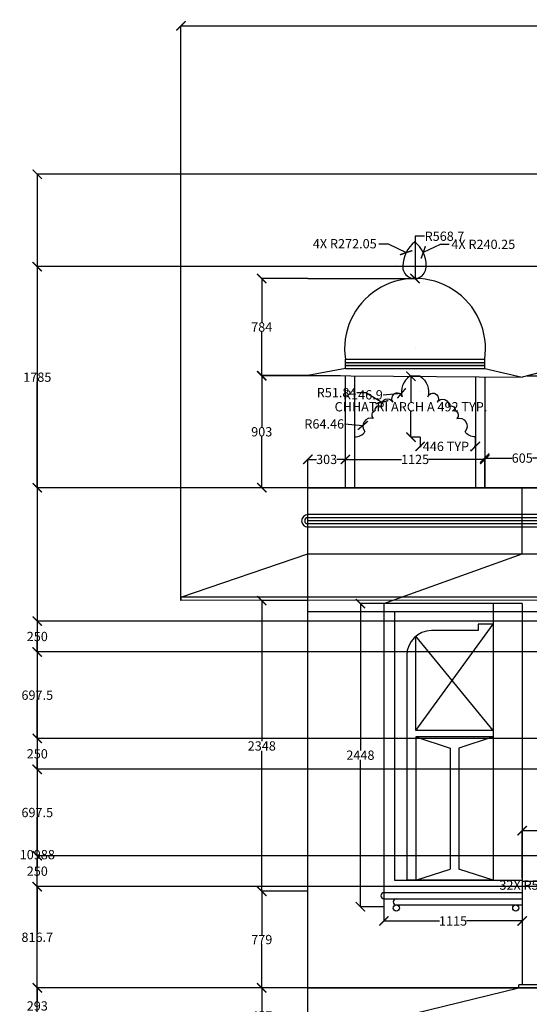
# Model space of a CAD drawing. Units: inches. Extents: x 829 to 33356404, y 1874 to 16983.
# Tile 3 of 9: x 844 to 4957, y 9032 to 16983. Entities that reach past the tile are written whole.
import ezdxf

# ---------------------------------------------------------------- set-up
doc = ezdxf.new("R2010")
doc.units = ezdxf.units.IN
doc.header["$MEASUREMENT"] = 0
doc.header["$PDMODE"] = 3
for name, color, linetype, lineweight in [('A-ANNO-DIMS', 2, 'Continuous', 18), ('A-ELEV', 7, 'Continuous', 25), ('A-ELEV-PATT', 8, 'Continuous', 13)]:
    doc.layers.add(name, color=color, linetype=linetype, lineweight=lineweight)
doc.styles.get("Standard").update_dxf_attribs({"font": 'arial.ttf'})
doc.dimstyles.get("Standard").update_dxf_attribs({"dimtxt": 75, "dimasz": 75, "dimexe": 0.18, "dimexo": 0.0625, "dimgap": 0.09, "dimtad": 0, "dimtih": 1, "dimtoh": 1, "dimdec": 0, "dimzin": 0, "dimdsep": 46, "dimtxsty": 'Standard', "dimblk": 'ARCHTICK', "dimcen": 0.09, "dimadec": 0, "dimazin": 0, "dimtfac": 1, "dimtdec": 0, "dimtofl": 0, "dimtmove": 0, "dimatfit": 3, "dimfxl": 1, "dimtolj": 1, "dimtzin": 0, "dimarcsym": 0})

# ---------------------------------------------------------------- blocks, each defined once
blk = doc.blocks.new('_ArchTick')
at = {"color": 0, "linetype": 'ByBlock', "const_width": 0.15}
blk.add_lwpolyline([(-0.5, -0.5), (0.5, 0.5)], dxfattribs=at)
blk = doc.blocks.new('*D7')
at = {"layer": 'A-ANNO-DIMS', "color": 0, "lineweight": -2, "transparency": 16777216}
for p, q in [((3169.7, 9165.5), (2797.3, 9165.5)), ((2797.5, 9165.5), (2797.5, 8975.2)), ((2797.5, 8708.5), (2797.5, 8898.7)), ((3169.7, 8708.5), (2797.3, 8708.5))]:
    blk.add_line(p, q, dxfattribs=at)
at = {"layer": 'Defpoints', "color": 0, "transparency": 16777216}
for p in [(3169.8, 9165.5), (2797.5, 8708.5), (3169.8, 8708.5)]:
    blk.add_point(p, dxfattribs=at)
at = {"layer": 'A-ANNO-DIMS', "color": 0, "lineweight": -2, "transparency": 16777216, "xscale": 75, "yscale": 75, "zscale": 75}
for p, rotation in [((2797.5, 9165.5), 90), ((2797.5, 8708.5), 270)]:
    blk.add_blockref('_ArchTick', p, dxfattribs=dict(at, rotation=rotation))
at = {"layer": 'A-ANNO-DIMS', "color": 0, "transparency": 16777216, "insert": (2797.5, 8937), "char_height": 75, "attachment_point": 5}
blk.add_mtext('\\A1;457', dxfattribs=at)
blk = doc.blocks.new('*D8')
at = {"layer": 'A-ANNO-DIMS', "color": 0, "lineweight": -2, "transparency": 16777216}
for p, q in [((3169.7, 9944.5), (2797.7, 9944.5)), ((2797.9, 9944.5), (2797.9, 9593.4)), ((2797.9, 9165.5), (2797.9, 9516.6)), ((3169.7, 9165.5), (2797.7, 9165.5))]:
    blk.add_line(p, q, dxfattribs=at)
at = {"layer": 'Defpoints', "color": 0, "transparency": 16777216}
for p in [(2797.9, 9944.5), (3169.8, 9944.5), (3169.8, 9165.5)]:
    blk.add_point(p, dxfattribs=at)
at = {"layer": 'A-ANNO-DIMS', "color": 0, "lineweight": -2, "transparency": 16777216, "xscale": 75, "yscale": 75, "zscale": 75}
for p, rotation in [((2797.9, 9944.5), 90), ((2797.9, 9165.5), 270)]:
    blk.add_blockref('_ArchTick', p, dxfattribs=dict(at, rotation=rotation))
at = {"layer": 'A-ANNO-DIMS', "color": 0, "transparency": 16777216, "insert": (2797.9, 9555), "char_height": 75, "attachment_point": 5}
blk.add_mtext('\\A1;779', dxfattribs=at)
blk = doc.blocks.new('*D9')
at = {"layer": 'A-ANNO-DIMS', "color": 0, "lineweight": -2, "transparency": 16777216}
for p, q in [((3169.7, 12292.5), (2797.7, 12292.5)), ((2797.9, 12292.5), (2797.9, 11156.9)), ((2797.9, 9944.5), (2797.9, 11080.1)), ((3169.7, 9944.5), (2797.7, 9944.5))]:
    blk.add_line(p, q, dxfattribs=at)
at = {"layer": 'Defpoints', "color": 0, "transparency": 16777216}
for p in [(2797.9, 12292.5), (3169.8, 12292.5), (3169.8, 9944.5)]:
    blk.add_point(p, dxfattribs=at)
at = {"layer": 'A-ANNO-DIMS', "color": 0, "lineweight": -2, "transparency": 16777216, "xscale": 75, "yscale": 75, "zscale": 75}
for p, rotation in [((2797.9, 12292.5), 90), ((2797.9, 9944.5), 270)]:
    blk.add_blockref('_ArchTick', p, dxfattribs=dict(at, rotation=rotation))
at = {"layer": 'A-ANNO-DIMS', "color": 0, "transparency": 16777216, "insert": (2797.9, 11118.5), "char_height": 75, "attachment_point": 5}
blk.add_mtext('\\A1;2348', dxfattribs=at)
blk = doc.blocks.new('*D40')
at = {"layer": 'A-ANNO-DIMS', "color": 0, "lineweight": -2, "transparency": 16777216}
for p, q in [((3784.1, 9884.2), (3784.1, 9704.8)), ((4899.1, 9819.4), (4899.1, 9704.8)), ((3784.1, 9705), (4232.8, 9705)), ((4899.1, 9705), (4450.4, 9705))]:
    blk.add_line(p, q, dxfattribs=at)
at = {"layer": 'Defpoints', "color": 0, "transparency": 16777216}
for p in [(3784.1, 9884.3), (4899.1, 9819.5), (3784.1, 9705)]:
    blk.add_point(p, dxfattribs=at)
at = {"layer": 'A-ANNO-DIMS', "color": 0, "lineweight": -2, "transparency": 16777216, "xscale": 75, "yscale": 75, "zscale": 75, "rotation": 180}
blk.add_blockref('_ArchTick', (3784.1, 9705), dxfattribs=at)
at = {"layer": 'A-ANNO-DIMS', "color": 0, "lineweight": -2, "transparency": 16777216, "xscale": 75, "yscale": 75, "zscale": 75}
blk.add_blockref('_ArchTick', (4899.1, 9705), dxfattribs=at)
at = {"layer": 'A-ANNO-DIMS', "color": 0, "transparency": 16777216, "insert": (4341.6, 9705), "char_height": 75, "attachment_point": 5}
blk.add_mtext('\\A1;1115', dxfattribs=at)
blk = doc.blocks.new('*D41')
at = {"layer": 'A-ANNO-DIMS', "color": 0, "lineweight": -2, "transparency": 16777216}
for p, q in [((3784, 12267.9), (3593.9, 12267.9)), ((3594.1, 12267.9), (3594.1, 11082.3)), ((3594.1, 9819.9), (3594.1, 11005.6)), ((3784, 9819.9), (3593.9, 9819.9))]:
    blk.add_line(p, q, dxfattribs=at)
at = {"layer": 'Defpoints', "color": 0, "transparency": 16777216}
for p in [(3594.1, 12267.9), (3784.1, 12267.9), (3784.1, 9819.9)]:
    blk.add_point(p, dxfattribs=at)
at = {"layer": 'A-ANNO-DIMS', "color": 0, "lineweight": -2, "transparency": 16777216, "xscale": 75, "yscale": 75, "zscale": 75}
for p, rotation in [((3594.1, 12267.9), 90), ((3594.1, 9819.9), 270)]:
    blk.add_blockref('_ArchTick', p, dxfattribs=dict(at, rotation=rotation))
at = {"layer": 'A-ANNO-DIMS', "color": 0, "transparency": 16777216, "insert": (3594.1, 11043.9), "char_height": 75, "attachment_point": 5}
blk.add_mtext('\\A1;2448', dxfattribs=at)
blk = doc.blocks.new('*D44')
at = {"layer": 'A-ANNO-DIMS', "color": 0, "lineweight": -2, "transparency": 16777216}
for p, q in [((4899.4, 10049.5), (4899.4, 10434.9)), ((4899.4, 10434.7), (5851.9, 10434.7)), ((7029.7, 10434.7), (6077.1, 10434.7)), ((7029.7, 10049.5), (7029.7, 10434.9))]:
    blk.add_line(p, q, dxfattribs=at)
at = {"layer": 'Defpoints', "color": 0, "transparency": 16777216}
for p in [(4899.4, 10434.7), (4899.4, 10049.4), (7029.7, 10049.4)]:
    blk.add_point(p, dxfattribs=at)
at = {"layer": 'A-ANNO-DIMS', "color": 0, "lineweight": -2, "transparency": 16777216, "xscale": 75, "yscale": 75, "zscale": 75, "rotation": 180}
blk.add_blockref('_ArchTick', (4899.4, 10434.7), dxfattribs=at)
at = {"layer": 'A-ANNO-DIMS', "color": 0, "lineweight": -2, "transparency": 16777216, "xscale": 75, "yscale": 75, "zscale": 75}
blk.add_blockref('_ArchTick', (7029.7, 10434.7), dxfattribs=at)
at = {"layer": 'A-ANNO-DIMS', "color": 0, "transparency": 16777216, "insert": (5964.5, 10434.7), "char_height": 75, "attachment_point": 5}
blk.add_mtext('\\A1;2130', dxfattribs=at)
blk = doc.blocks.new('*D46')
at = {"layer": 'A-ANNO-DIMS', "color": 0, "lineweight": -2, "transparency": 16777216}
for p, q in [((3472.8, 13262.8), (3472.8, 13432.5)), ((3472.8, 13432.3), (3926.4, 13432.3)), ((4597.8, 13432.3), (4144.1, 13432.3)), ((4597.8, 13262.8), (4597.8, 13432.5))]:
    blk.add_line(p, q, dxfattribs=at)
at = {"layer": 'Defpoints', "color": 0, "transparency": 16777216}
for p in [(4597.8, 13432.3), (3472.8, 13262.7), (4597.8, 13262.7)]:
    blk.add_point(p, dxfattribs=at)
at = {"layer": 'A-ANNO-DIMS', "color": 0, "lineweight": -2, "transparency": 16777216, "xscale": 75, "yscale": 75, "zscale": 75, "rotation": 180}
blk.add_blockref('_ArchTick', (3472.8, 13432.3), dxfattribs=at)
at = {"layer": 'A-ANNO-DIMS', "color": 0, "lineweight": -2, "transparency": 16777216, "xscale": 75, "yscale": 75, "zscale": 75}
blk.add_blockref('_ArchTick', (4597.8, 13432.3), dxfattribs=at)
at = {"layer": 'A-ANNO-DIMS', "color": 0, "transparency": 16777216, "insert": (4035.3, 13432.3), "char_height": 75, "attachment_point": 5}
blk.add_mtext('\\A1;1125', dxfattribs=at)
blk = doc.blocks.new('*D47')
at = {"layer": 'A-ANNO-DIMS', "color": 0, "lineweight": -2, "transparency": 16777216}
for p, q in [((4597.8, 13204.1), (4597.8, 13443.2)), ((4597.8, 13443), (4816.8, 13443)), ((5202.8, 13443), (4983.7, 13443)), ((5202.8, 13204.1), (5202.8, 13443.2))]:
    blk.add_line(p, q, dxfattribs=at)
at = {"layer": 'Defpoints', "color": 0, "transparency": 16777216}
for p in [(5202.8, 13443), (4597.8, 13204), (5202.8, 13204)]:
    blk.add_point(p, dxfattribs=at)
at = {"layer": 'A-ANNO-DIMS', "color": 0, "lineweight": -2, "transparency": 16777216, "xscale": 75, "yscale": 75, "zscale": 75, "rotation": 180}
blk.add_blockref('_ArchTick', (4597.8, 13443), dxfattribs=at)
at = {"layer": 'A-ANNO-DIMS', "color": 0, "lineweight": -2, "transparency": 16777216, "xscale": 75, "yscale": 75, "zscale": 75}
blk.add_blockref('_ArchTick', (5202.8, 13443), dxfattribs=at)
at = {"layer": 'A-ANNO-DIMS', "color": 0, "transparency": 16777216, "insert": (4900.3, 13443), "char_height": 75, "attachment_point": 5}
blk.add_mtext('\\A1;605', dxfattribs=at)
blk = doc.blocks.new('*D57')
at = {"layer": 'A-ANNO-DIMS', "color": 0, "lineweight": -2, "transparency": 16777216}
for p, q in [((3433.5, 14107.2), (2797.3, 14107.2)), ((2797.5, 14107.2), (2797.5, 13694)), ((2797.5, 13204), (2797.5, 13617.2)), ((3472.7, 13204), (2797.3, 13204))]:
    blk.add_line(p, q, dxfattribs=at)
at = {"layer": 'Defpoints', "color": 0, "transparency": 16777216}
for p in [(2797.5, 14107.2), (3433.5, 14107.2), (3472.8, 13204)]:
    blk.add_point(p, dxfattribs=at)
at = {"layer": 'A-ANNO-DIMS', "color": 0, "lineweight": -2, "transparency": 16777216, "xscale": 75, "yscale": 75, "zscale": 75}
for p, rotation in [((2797.5, 14107.2), 90), ((2797.5, 13204), 270)]:
    blk.add_blockref('_ArchTick', p, dxfattribs=dict(at, rotation=rotation))
at = {"layer": 'A-ANNO-DIMS', "color": 0, "transparency": 16777216, "insert": (2797.5, 13655.6), "char_height": 75, "attachment_point": 5}
blk.add_mtext('\\A1;903', dxfattribs=at)
blk = doc.blocks.new('*D68')
at = {"layer": 'A-ANNO-DIMS', "color": 0, "lineweight": -2, "transparency": 16777216}
for p, q in [((3169.7, 14893.2), (2797.2, 14893.2)), ((2797.3, 14893.2), (2797.3, 14539.6)), ((2797.3, 14109.2), (2797.3, 14462.8)), ((3169.7, 14109.2), (2797.2, 14109.2))]:
    blk.add_line(p, q, dxfattribs=at)
at = {"layer": 'Defpoints', "color": 0, "transparency": 16777216}
for p in [(2797.3, 14893.2), (3169.8, 14893.2), (3169.8, 14109.2)]:
    blk.add_point(p, dxfattribs=at)
at = {"layer": 'A-ANNO-DIMS', "color": 0, "lineweight": -2, "transparency": 16777216, "xscale": 75, "yscale": 75, "zscale": 75}
for p, rotation in [((2797.3, 14893.2), 90), ((2797.3, 14109.2), 270)]:
    blk.add_blockref('_ArchTick', p, dxfattribs=dict(at, rotation=rotation))
at = {"layer": 'A-ANNO-DIMS', "color": 0, "transparency": 16777216, "insert": (2797.3, 14501.2), "char_height": 75, "attachment_point": 5}
blk.add_mtext('\\A1;784', dxfattribs=at)
blk = doc.blocks.new('*D69')
at = {"layer": 'A-ANNO-DIMS', "color": 0, "lineweight": -2, "transparency": 16777216}
for p, q in [((3169.8, 13204.1), (3169.8, 13432.7)), ((3169.8, 13432.5), (3238.4, 13432.5)), ((3472.8, 13432.5), (3404.2, 13432.5)), ((3472.8, 13204.1), (3472.8, 13432.7))]:
    blk.add_line(p, q, dxfattribs=at)
at = {"layer": 'Defpoints', "color": 0, "transparency": 16777216}
for p in [(3472.8, 13432.5), (3169.8, 13204), (3472.8, 13204)]:
    blk.add_point(p, dxfattribs=at)
at = {"layer": 'A-ANNO-DIMS', "color": 0, "lineweight": -2, "transparency": 16777216, "xscale": 75, "yscale": 75, "zscale": 75, "rotation": 180}
blk.add_blockref('_ArchTick', (3169.8, 13432.5), dxfattribs=at)
at = {"layer": 'A-ANNO-DIMS', "color": 0, "lineweight": -2, "transparency": 16777216, "xscale": 75, "yscale": 75, "zscale": 75}
blk.add_blockref('_ArchTick', (3472.8, 13432.5), dxfattribs=at)
at = {"layer": 'A-ANNO-DIMS', "color": 0, "transparency": 16777216, "insert": (3321.3, 13432.5), "char_height": 75, "attachment_point": 5}
blk.add_mtext('\\A1;303', dxfattribs=at)
blk = doc.blocks.new('CHHATRI-ARCH-A')
blk.add_lwpolyline([(0, 0.5, 0.306755), (82.5, 43.8, 10.100933)], format="xyb")
for centre, radius, start, end in [((524.9, 364.6), 146.9, 122.41425, 196.90759), ((342.3, 308.5), 44.1, 17.62677, 218.36127), ((195.1, 217.8), 31.7, 54.88866, 193.78992), ((264.3, 252.9), 51.8, 32.98834, 190.27791), ((174.5, 175.2), 36.4, 106.30777, 227.87761), ((130.5, 86.8), 64.5, 72.31695, 221.86505)]:
    blk.add_arc(centre, radius, start, end)
blk = doc.blocks.new('*D74')
at = {"layer": 'A-ANNO-DIMS', "color": 0, "lineweight": -2, "transparency": 16777216}
for p, q in [((4075.9, 14103.5), (4002, 14103.6)), ((4002.1, 14103.6), (4002, 13896.5)), ((4001.8, 13611.6), (4001.9, 13818.7)), ((4075.5, 13611.6), (4001.6, 13611.6))]:
    blk.add_line(p, q, dxfattribs=at)
at = {"layer": 'Defpoints', "color": 0, "transparency": 16777216}
for p in [(4002.1, 14103.6), (4075.9, 14103.5), (4075.6, 13611.6)]:
    blk.add_point(p, dxfattribs=at)
at = {"layer": 'A-ANNO-DIMS', "color": 0, "lineweight": -2, "transparency": 16777216, "xscale": 75, "yscale": 75, "zscale": 75}
for p, rotation in [((4002.1, 14103.6), 89.95904466512309), ((4001.8, 13611.6), 269.9590446651231)]:
    blk.add_blockref('_ArchTick', p, dxfattribs=dict(at, rotation=rotation))
at = {"layer": 'A-ANNO-DIMS', "color": 0, "transparency": 16777216, "insert": (4002, 13857.6), "char_height": 75, "attachment_point": 5}
blk.add_mtext('\\A1;CHHATRI ARCH A 492 TYP.', dxfattribs=at)
blk = doc.blocks.new('*D75')
at = {"layer": 'A-ANNO-DIMS', "color": 0, "lineweight": -2, "transparency": 16777216}
for p, q in [((4075.6, 13611.5), (4075.5, 13537.6)), ((4521.7, 13611.2), (4521.7, 13537.3)), ((4075.5, 13537.8), (4085.3, 13537.8)), ((4521.7, 13537.5), (4511.9, 13537.5))]:
    blk.add_line(p, q, dxfattribs=at)
at = {"layer": 'Defpoints', "color": 0, "transparency": 16777216}
for p in [(4075.6, 13611.6), (4521.7, 13611.3), (4075.5, 13537.8)]:
    blk.add_point(p, dxfattribs=at)
at = {"layer": 'A-ANNO-DIMS', "color": 0, "lineweight": -2, "transparency": 16777216, "xscale": 75, "yscale": 75, "zscale": 75}
for p, rotation in [((4075.5, 13537.8), 179.959044665123), ((4521.7, 13537.5), 359.959044665123)]:
    blk.add_blockref('_ArchTick', p, dxfattribs=dict(at, rotation=rotation))
at = {"layer": 'A-ANNO-DIMS', "color": 0, "transparency": 16777216, "insert": (4298.6, 13537.6), "char_height": 75, "attachment_point": 5}
blk.add_mtext('\\A1;446 TYP.', dxfattribs=at)
blk = doc.blocks.new('*D82')
at = {"layer": 'A-ANNO-DIMS', "color": 0, "lineweight": -2, "transparency": 16777216}
for p, q in [((2145.7, 12292.3), (2145.7, 16934.2)), ((2145.7, 16934), (13417.9, 16934)), ((24973.9, 16934), (13701.7, 16934)), ((24973.9, 12320.9), (24973.9, 16934.2))]:
    blk.add_line(p, q, dxfattribs=at)
at = {"layer": 'Defpoints', "color": 0, "transparency": 16777216}
for p in [(24973.9, 16934), (2145.7, 12292.2), (24973.9, 12320.9)]:
    blk.add_point(p, dxfattribs=at)
at = {"layer": 'A-ANNO-DIMS', "color": 0, "lineweight": -2, "transparency": 16777216, "xscale": 75, "yscale": 75, "zscale": 75, "rotation": 180}
blk.add_blockref('_ArchTick', (2145.7, 16934), dxfattribs=at)
at = {"layer": 'A-ANNO-DIMS', "color": 0, "lineweight": -2, "transparency": 16777216, "xscale": 75, "yscale": 75, "zscale": 75}
blk.add_blockref('_ArchTick', (24973.9, 16934), dxfattribs=at)
at = {"layer": 'A-ANNO-DIMS', "color": 0, "transparency": 16777216, "insert": (13559.8, 16934), "char_height": 75, "attachment_point": 5}
blk.add_mtext('\\A1;22828', dxfattribs=at)
blk = doc.blocks.new('*D83')
at = {"layer": 'A-ANNO-DIMS', "color": 0, "lineweight": -2, "transparency": 16777216}
for p, q in [((13604.5, 15734.9), (985.4, 15734.9)), ((985.6, 15734.9), (985.6, 10279.1)), ((985.6, 4746.5), (985.6, 10202.3)), ((3169.7, 4746.5), (985.4, 4746.5))]:
    blk.add_line(p, q, dxfattribs=at)
at = {"layer": 'Defpoints', "color": 0, "transparency": 16777216}
for p in [(985.6, 15734.9), (13604.5, 15734.9), (3169.8, 4746.5)]:
    blk.add_point(p, dxfattribs=at)
at = {"layer": 'A-ANNO-DIMS', "color": 0, "lineweight": -2, "transparency": 16777216, "xscale": 75, "yscale": 75, "zscale": 75}
for p, rotation in [((985.6, 15734.9), 90), ((985.6, 4746.5), 270)]:
    blk.add_blockref('_ArchTick', p, dxfattribs=dict(at, rotation=rotation))
at = {"layer": 'A-ANNO-DIMS', "color": 0, "transparency": 16777216, "insert": (985.6, 10240.7), "char_height": 75, "attachment_point": 5}
blk.add_mtext('\\A1;10988', dxfattribs=at)
blk = doc.blocks.new('*D84')
at = {"layer": 'A-ANNO-DIMS', "color": 0, "lineweight": -2, "transparency": 16777216}
for p, q in [((12044.3, 14988.9), (985.4, 14988.9)), ((985.6, 14988.9), (985.6, 14134.8)), ((985.6, 13204), (985.6, 14058.1)), ((9930.7, 13204), (985.4, 13204))]:
    blk.add_line(p, q, dxfattribs=at)
at = {"layer": 'Defpoints', "color": 0, "transparency": 16777216}
for p in [(985.6, 14988.9), (12044.4, 14988.9), (9930.8, 13204)]:
    blk.add_point(p, dxfattribs=at)
at = {"layer": 'A-ANNO-DIMS', "color": 0, "lineweight": -2, "transparency": 16777216, "xscale": 75, "yscale": 75, "zscale": 75}
for p, rotation in [((985.6, 14988.9), 90), ((985.6, 13204), 270)]:
    blk.add_blockref('_ArchTick', p, dxfattribs=dict(at, rotation=rotation))
at = {"layer": 'A-ANNO-DIMS', "color": 0, "transparency": 16777216, "insert": (985.6, 14096.5), "char_height": 75, "attachment_point": 5}
blk.add_mtext('\\A1;1785', dxfattribs=at)
blk = doc.blocks.new('*D98')
at = {"layer": 'A-ANNO-DIMS', "color": 0, "lineweight": -2, "transparency": 16777216}
for p, q in [((9793.7, 9165.5), (985.4, 9165.5)), ((985.6, 9165.5), (985.6, 9057.4)), ((985.6, 8872.5), (985.6, 8980.6)), ((9793.7, 8872.5), (985.4, 8872.5))]:
    blk.add_line(p, q, dxfattribs=at)
at = {"layer": 'Defpoints', "color": 0, "transparency": 16777216}
for p in [(985.6, 9165.5), (9793.7, 9165.5), (9793.7, 8872.5)]:
    blk.add_point(p, dxfattribs=at)
at = {"layer": 'A-ANNO-DIMS', "color": 0, "lineweight": -2, "transparency": 16777216, "xscale": 75, "yscale": 75, "zscale": 75}
for p, rotation in [((985.6, 9165.5), 90), ((985.6, 8872.5), 270)]:
    blk.add_blockref('_ArchTick', p, dxfattribs=dict(at, rotation=rotation))
at = {"layer": 'A-ANNO-DIMS', "color": 0, "transparency": 16777216, "insert": (985.6, 9019), "char_height": 75, "attachment_point": 5}
blk.add_mtext('\\A1;293', dxfattribs=at)
blk = doc.blocks.new('*D99')
at = {"layer": 'A-ANNO-DIMS', "color": 0, "lineweight": -2, "transparency": 16777216}
for p, q in [((9793.7, 9982.2), (985.4, 9982.2)), ((985.6, 9982.2), (985.6, 9612.2)), ((985.6, 9165.5), (985.6, 9535.4)), ((9793.7, 9165.5), (985.4, 9165.5))]:
    blk.add_line(p, q, dxfattribs=at)
at = {"layer": 'Defpoints', "color": 0, "transparency": 16777216}
for p in [(985.6, 9982.2), (9793.7, 9982.2), (9793.7, 9165.5)]:
    blk.add_point(p, dxfattribs=at)
at = {"layer": 'A-ANNO-DIMS', "color": 0, "lineweight": -2, "transparency": 16777216, "xscale": 75, "yscale": 75, "zscale": 75}
for p, rotation in [((985.6, 9982.2), 90), ((985.6, 9165.5), 270)]:
    blk.add_blockref('_ArchTick', p, dxfattribs=dict(at, rotation=rotation))
at = {"layer": 'A-ANNO-DIMS', "color": 0, "transparency": 16777216, "insert": (985.6, 9573.8), "char_height": 75, "attachment_point": 5}
blk.add_mtext('\\A1;816.7', dxfattribs=at)
blk = doc.blocks.new('*D100')
at = {"layer": 'A-ANNO-DIMS', "color": 0, "lineweight": -2, "transparency": 16777216}
for p, q in [((9829.1, 10232.2), (985.4, 10232.2)), ((985.6, 10232.2), (985.6, 10145.6)), ((985.6, 9982.2), (985.6, 10068.8)), ((9793.7, 9982.2), (985.4, 9982.2))]:
    blk.add_line(p, q, dxfattribs=at)
at = {"layer": 'Defpoints', "color": 0, "transparency": 16777216}
for p in [(985.6, 10232.2), (9829.2, 10232.2), (9793.7, 9982.2)]:
    blk.add_point(p, dxfattribs=at)
at = {"layer": 'A-ANNO-DIMS', "color": 0, "lineweight": -2, "transparency": 16777216, "xscale": 75, "yscale": 75, "zscale": 75}
for p, rotation in [((985.6, 10232.2), 90), ((985.6, 9982.2), 270)]:
    blk.add_blockref('_ArchTick', p, dxfattribs=dict(at, rotation=rotation))
at = {"layer": 'A-ANNO-DIMS', "color": 0, "transparency": 16777216, "insert": (985.6, 10107.2), "char_height": 75, "attachment_point": 5}
blk.add_mtext('\\A1;250', dxfattribs=at)
blk = doc.blocks.new('*D101')
at = {"layer": 'A-ANNO-DIMS', "color": 0, "lineweight": -2, "transparency": 16777216}
for p, q in [((9829.1, 10929.7), (985.4, 10929.7)), ((985.6, 10929.7), (985.6, 10619.3)), ((985.6, 10232.2), (985.6, 10542.6)), ((9829.1, 10232.2), (985.4, 10232.2))]:
    blk.add_line(p, q, dxfattribs=at)
at = {"layer": 'Defpoints', "color": 0, "transparency": 16777216}
for p in [(985.6, 10929.7), (9829.2, 10929.7), (9829.2, 10232.2)]:
    blk.add_point(p, dxfattribs=at)
at = {"layer": 'A-ANNO-DIMS', "color": 0, "lineweight": -2, "transparency": 16777216, "xscale": 75, "yscale": 75, "zscale": 75}
for p, rotation in [((985.6, 10929.7), 90), ((985.6, 10232.2), 270)]:
    blk.add_blockref('_ArchTick', p, dxfattribs=dict(at, rotation=rotation))
at = {"layer": 'A-ANNO-DIMS', "color": 0, "transparency": 16777216, "insert": (985.6, 10580.9), "char_height": 75, "attachment_point": 5}
blk.add_mtext('\\A1;697.5', dxfattribs=at)
blk = doc.blocks.new('*D102')
at = {"layer": 'A-ANNO-DIMS', "color": 0, "lineweight": -2, "transparency": 16777216}
for p, q in [((9829.1, 11179.7), (985.4, 11179.7)), ((985.6, 11179.7), (985.6, 11093.1)), ((985.6, 10929.7), (985.6, 11016.3)), ((9829.1, 10929.7), (985.4, 10929.7))]:
    blk.add_line(p, q, dxfattribs=at)
at = {"layer": 'Defpoints', "color": 0, "transparency": 16777216}
for p in [(985.6, 11179.7), (9829.2, 11179.7), (9829.2, 10929.7)]:
    blk.add_point(p, dxfattribs=at)
at = {"layer": 'A-ANNO-DIMS', "color": 0, "lineweight": -2, "transparency": 16777216, "xscale": 75, "yscale": 75, "zscale": 75}
for p, rotation in [((985.6, 11179.7), 90), ((985.6, 10929.7), 270)]:
    blk.add_blockref('_ArchTick', p, dxfattribs=dict(at, rotation=rotation))
at = {"layer": 'A-ANNO-DIMS', "color": 0, "transparency": 16777216, "insert": (985.6, 11054.7), "char_height": 75, "attachment_point": 5}
blk.add_mtext('\\A1;250', dxfattribs=at)
blk = doc.blocks.new('*D103')
at = {"layer": 'A-ANNO-DIMS', "color": 0, "lineweight": -2, "transparency": 16777216}
for p, q in [((9829.1, 11877.2), (985.4, 11877.2)), ((985.6, 11877.2), (985.6, 11566.8)), ((985.6, 11179.7), (985.6, 11490.1)), ((9829.1, 11179.7), (985.4, 11179.7))]:
    blk.add_line(p, q, dxfattribs=at)
at = {"layer": 'Defpoints', "color": 0, "transparency": 16777216}
for p in [(985.6, 11877.2), (9829.2, 11877.2), (9829.2, 11179.7)]:
    blk.add_point(p, dxfattribs=at)
at = {"layer": 'A-ANNO-DIMS', "color": 0, "lineweight": -2, "transparency": 16777216, "xscale": 75, "yscale": 75, "zscale": 75}
for p, rotation in [((985.6, 11877.2), 90), ((985.6, 11179.7), 270)]:
    blk.add_blockref('_ArchTick', p, dxfattribs=dict(at, rotation=rotation))
at = {"layer": 'A-ANNO-DIMS', "color": 0, "transparency": 16777216, "insert": (985.6, 11528.5), "char_height": 75, "attachment_point": 5}
blk.add_mtext('\\A1;697.5', dxfattribs=at)
blk = doc.blocks.new('*D104')
at = {"layer": 'A-ANNO-DIMS', "color": 0, "lineweight": -2, "transparency": 16777216}
for p, q in [((9559.8, 12127.2), (985.4, 12127.2)), ((985.6, 12127.2), (985.6, 12040.6)), ((985.6, 11877.2), (985.6, 11963.8)), ((9829.1, 11877.2), (985.4, 11877.2))]:
    blk.add_line(p, q, dxfattribs=at)
at = {"layer": 'Defpoints', "color": 0, "transparency": 16777216}
for p in [(985.6, 12127.2), (9559.8, 12127.2), (9829.2, 11877.2)]:
    blk.add_point(p, dxfattribs=at)
at = {"layer": 'A-ANNO-DIMS', "color": 0, "lineweight": -2, "transparency": 16777216, "xscale": 75, "yscale": 75, "zscale": 75}
for p, rotation in [((985.6, 12127.2), 90), ((985.6, 11877.2), 270)]:
    blk.add_blockref('_ArchTick', p, dxfattribs=dict(at, rotation=rotation))
at = {"layer": 'A-ANNO-DIMS', "color": 0, "transparency": 16777216, "insert": (985.6, 12002.2), "char_height": 75, "attachment_point": 5}
blk.add_mtext('\\A1;250', dxfattribs=at)
blk = doc.blocks.new('*D114')
at = {"layer": 'A-ANNO-DIMS', "color": 0, "lineweight": -2, "transparency": 16777216}
for p, q in [((5159.5, 9994.8), (5234.5, 9994.8)), ((5234.5, 9994.8), (5509.2, 9839.5)), ((5967, 9580.4), (5967, 9580.6)), ((5967, 9580.5), (5967.1, 9580.5))]:
    blk.add_line(p, q, dxfattribs=at)
at = {"layer": 'Defpoints', "color": 0, "transparency": 16777216}
for p in [(5509.2, 9839.5), (5967, 9580.5)]:
    blk.add_point(p, dxfattribs=at)
at = {"layer": 'A-ANNO-DIMS', "color": 0, "lineweight": -2, "transparency": 16777216, "xscale": 75, "yscale": 75, "zscale": 75, "rotation": 330.5044086003726}
blk.add_blockref('_ArchTick', (5509.2, 9839.5), dxfattribs=at)
at = {"layer": 'A-ANNO-DIMS', "color": 0, "transparency": 16777216, "insert": (4931.1, 9994.8), "char_height": 75, "attachment_point": 5}
blk.add_mtext('\\A1;32X R526', dxfattribs=at)
blk = doc.blocks.new('*D116')
at = {"layer": 'A-ANNO-DIMS', "color": 0, "lineweight": -2, "transparency": 16777216}
for p, q in [((4110.3, 15234.8), (4035.3, 15234.8)), ((4035.3, 15234.8), (4035.3, 14893.5)), ((4035.2, 14324.8), (4035.4, 14324.8)), ((4035.3, 14324.7), (4035.3, 14324.9))]:
    blk.add_line(p, q, dxfattribs=at)
at = {"layer": 'Defpoints', "color": 0, "transparency": 16777216}
for p in [(4035.3, 14893.5), (4035.3, 14324.8)]:
    blk.add_point(p, dxfattribs=at)
at = {"layer": 'A-ANNO-DIMS', "color": 0, "lineweight": -2, "transparency": 16777216, "xscale": 75, "yscale": 75, "zscale": 75, "rotation": 270}
blk.add_blockref('_ArchTick', (4035.3, 14893.5), dxfattribs=at)
at = {"layer": 'A-ANNO-DIMS', "color": 0, "transparency": 16777216, "insert": (4272.8, 15234.8), "char_height": 75, "attachment_point": 5}
blk.add_mtext('\\A1;R568.7', dxfattribs=at)
blk = doc.blocks.new('*D118')
at = {"layer": 'A-ANNO-DIMS', "color": 0, "lineweight": -2, "transparency": 16777216}
for p, q in [((3741.8, 15174.1), (3816.8, 15174.1)), ((3816.8, 15174.1), (3963.2, 15102)), ((4207.2, 14981.8), (4207.4, 14981.8)), ((4207.3, 14981.7), (4207.3, 14981.9))]:
    blk.add_line(p, q, dxfattribs=at)
at = {"layer": 'Defpoints', "color": 0, "transparency": 16777216}
for p in [(3963.2, 15102), (4207.3, 14981.8)]:
    blk.add_point(p, dxfattribs=at)
at = {"layer": 'A-ANNO-DIMS', "color": 0, "lineweight": -2, "transparency": 16777216, "xscale": 75, "yscale": 75, "zscale": 75, "rotation": 333.7791699204543}
blk.add_blockref('_ArchTick', (3963.2, 15102), dxfattribs=at)
at = {"layer": 'A-ANNO-DIMS', "color": 0, "transparency": 16777216, "insert": (3467.8, 15174.1), "char_height": 75, "attachment_point": 5}
blk.add_mtext('\\A1;4X R272.05', dxfattribs=at)
blk = doc.blocks.new('*D119')
at = {"layer": 'A-ANNO-DIMS', "color": 0, "lineweight": -2, "transparency": 16777216}
for p, q in [((4236.7, 15168.9), (4101.4, 15104.3)), ((4311.7, 15168.9), (4236.7, 15168.9)), ((3884.5, 15000.7), (3884.7, 15000.7)), ((3884.6, 15000.7), (3884.6, 15000.8))]:
    blk.add_line(p, q, dxfattribs=at)
at = {"layer": 'Defpoints', "color": 0, "transparency": 16777216}
for p in [(4101.4, 15104.3), (3884.6, 15000.7)]:
    blk.add_point(p, dxfattribs=at)
at = {"layer": 'A-ANNO-DIMS', "color": 0, "lineweight": -2, "transparency": 16777216, "xscale": 75, "yscale": 75, "zscale": 75, "rotation": 205.5314683361511}
blk.add_blockref('_ArchTick', (4101.4, 15104.3), dxfattribs=at)
at = {"layer": 'A-ANNO-DIMS', "color": 0, "transparency": 16777216, "insert": (4585.8, 15168.9), "char_height": 75, "attachment_point": 5}
blk.add_mtext('\\A1;4X R240.25', dxfattribs=at)
blk = doc.blocks.new('*D120')
at = {"layer": 'A-ANNO-DIMS', "color": 0, "lineweight": -2, "transparency": 16777216}
for p, q in [((3464.5, 13718.8), (3614, 13706.7)), ((3678.2, 13701.5), (3678.4, 13701.5)), ((3678.3, 13701.4), (3678.3, 13701.6))]:
    blk.add_line(p, q, dxfattribs=at)
at = {"layer": 'Defpoints', "color": 0, "transparency": 16777216}
for p in [(3614, 13706.7), (3678.3, 13701.5)]:
    blk.add_point(p, dxfattribs=at)
at = {"layer": 'A-ANNO-DIMS', "color": 0, "lineweight": -2, "transparency": 16777216, "xscale": 75, "yscale": 75, "zscale": 75, "rotation": 355.3684214506782}
blk.add_blockref('_ArchTick', (3614, 13706.7), dxfattribs=at)
at = {"layer": 'A-ANNO-DIMS', "color": 0, "transparency": 16777216, "insert": (3302, 13718.8), "char_height": 75, "attachment_point": 5}
blk.add_mtext('\\A1;R64.46', dxfattribs=at)
blk = doc.blocks.new('*D121')
at = {"layer": 'A-ANNO-DIMS', "color": 0, "lineweight": -2, "transparency": 16777216}
for p, q in [((3564.1, 13971.8), (3639.1, 13971.8)), ((3639.1, 13971.8), (3767.7, 13894.4)), ((3812, 13867.7), (3812.2, 13867.7)), ((3812.1, 13867.6), (3812.1, 13867.8))]:
    blk.add_line(p, q, dxfattribs=at)
at = {"layer": 'Defpoints', "color": 0, "transparency": 16777216}
for p in [(3767.7, 13894.4), (3812.1, 13867.7)]:
    blk.add_point(p, dxfattribs=at)
at = {"layer": 'A-ANNO-DIMS', "color": 0, "lineweight": -2, "transparency": 16777216, "xscale": 75, "yscale": 75, "zscale": 75, "rotation": 328.9536985471738}
blk.add_blockref('_ArchTick', (3767.7, 13894.4), dxfattribs=at)
at = {"layer": 'A-ANNO-DIMS', "color": 0, "transparency": 16777216, "insert": (3401.8, 13971.8), "char_height": 75, "attachment_point": 5}
blk.add_mtext('\\A1;R51.84', dxfattribs=at)
blk = doc.blocks.new('*D122')
at = {"layer": 'A-ANNO-DIMS', "color": 0, "lineweight": -2, "transparency": 16777216}
for p, q in [((3776.8, 13954), (3926.3, 13966.8)), ((4072.6, 13979.3), (4072.7, 13979.3)), ((4072.7, 13979.2), (4072.7, 13979.4))]:
    blk.add_line(p, q, dxfattribs=at)
at = {"layer": 'Defpoints', "color": 0, "transparency": 16777216}
for p in [(3926.3, 13966.8), (4072.7, 13979.3)]:
    blk.add_point(p, dxfattribs=at)
at = {"layer": 'A-ANNO-DIMS', "color": 0, "lineweight": -2, "transparency": 16777216, "xscale": 75, "yscale": 75, "zscale": 75, "rotation": 4.896573162215946}
blk.add_blockref('_ArchTick', (3926.3, 13966.8), dxfattribs=at)
at = {"layer": 'A-ANNO-DIMS', "color": 0, "transparency": 16777216, "insert": (3614.3, 13954), "char_height": 75, "attachment_point": 5}
blk.add_mtext('\\A1;R146.9', dxfattribs=at)

msp = doc.modelspace()

# ---------------------------------------------------------------- hatches: boundary and pattern name
at = {"layer": 'A-ELEV-PATT'}
h = msp.add_hatch(color=256, dxfattribs=at)
h.dxf.hatch_style = 1
h.paths.add_polyline_path([(4035.278, 14215.703), (3472.778, 14215.703), (3472.778, 14190.703), (4035.278, 14190.703)])
h = msp.add_hatch(color=256, dxfattribs=at)
h.dxf.hatch_style = 1
h.paths.add_polyline_path([(4597.778, 14215.703), (4035.278, 14215.703), (4035.278, 14190.703), (4597.778, 14190.703)])

# ---------------------------------------------------------------- linework, layer by layer
at = {"layer": 'A-ELEV'}
for p, q in [((3169.778, 14893.194), (4054.603, 14893.194)), ((3472.778, 14240.703), (4597.778, 14240.703)), ((3472.778, 14165.703), (3472.778, 14240.703)), ((4597.778, 14165.703), (4597.778, 14240.703)), ((3472.778, 14165.703), (3169.778, 14109.194)), ((3472.778, 14215.703), (4597.778, 14215.703)), ((3472.778, 14190.703), (4597.778, 14190.703)), ((3472.778, 14165.703), (4597.778, 14165.703)), ((4597.778, 14165.703), (4899.778, 14096.847)), ((5202.778, 14176.035), (4899.778, 14096.847)), ((3169.778, 14109.194), (4899.778, 14096.847)), ((3472.778, 13204.032), (3472.778, 14107.032)), ((3547.778, 13204.032), (3547.778, 14106.496)), ((4522.778, 14099.537), (4522.778, 13204.032)), ((4597.778, 14099.002), (4597.778, 13204.032)), ((4939.313, 14107.179), (6629.778, 14107.179)), ((3169.778, 9944.468), (3169.778, 13204.032)), ((3169.778, 13204.032), (23949.778, 13204.032)), ((4900.278, 12669.032), (4900.278, 13204.032)), ((23949.778, 12986.532), (3169.778, 12986.532)), ((23949.778, 12961.532), (3169.778, 12961.532)), ((23949.778, 12936.532), (3169.778, 12936.532)), ((23949.778, 12911.532), (3169.778, 12911.532)), ((23949.778, 12886.532), (3169.778, 12886.532)), ((2145.628, 12320.882), (3169.778, 12669.032)), ((3169.778, 12669.032), (23949.778, 12669.032)), ((3784.097, 12267.948), (4900.278, 12669.032)), ((24973.929, 12320.882), (2145.628, 12320.882)), ((2145.628, 12320.882), (2145.651, 12292.214)), ((24973.929, 12310.744), (2145.651, 12292.214)), ((4899.383, 12267.948), (3784.097, 12267.948)), ((3784.097, 12267.948), (3784.097, 9819.948)), ((4665.591, 12267.948), (4665.591, 10034.257)), ((4899.383, 12267.948), (4899.383, 9188.877)), ((22522.278, 12202.212), (3169.778, 12202.212)), ((4665.591, 12202.212), (3868.626, 12202.212)), ((3868.626, 12202.212), (3868.626, 10034.257)), ((4040.202, 11242.683), (4665.591, 12100.687)), ((4665.591, 12100.687), (4544.777, 12100.687)), ((4544.777, 12100.687), (4544.777, 12049.925)), ((4665.591, 12100.687), (4665.591, 12100.687)), ((4544.777, 12049.925), (4168.626, 12049.925)), ((4544.777, 12049.925), (4544.777, 12049.925)), ((4040.225, 11242.683), (4040.225, 12004.367)), ((4665.591, 11242.683), (4041.959, 12004.701)), ((3968.626, 11849.925), (3968.626, 11754.206)), ((3968.626, 11806.442), (3968.626, 10034.257)), ((4665.591, 11242.683), (4040.202, 11242.683)), ((4665.591, 11242.683), (4665.591, 11242.683)), ((4665.591, 11191.921), (4040.202, 11191.921)), ((4040.202, 11191.921), (4317.363, 11101.847)), ((4040.202, 11191.921), (4040.202, 10034.257)), ((4665.591, 11191.921), (4388.43, 11101.847)), ((4317.363, 11101.847), (4317.363, 10124.33)), ((4388.43, 11101.847), (4388.43, 10124.33)), ((4040.202, 10034.257), (4317.363, 10124.33)), ((4665.591, 10034.257), (4388.43, 10124.33)), ((3868.626, 10034.257), (4899.097, 10034.257)), ((4643.501, 10034.257), (3967.349, 10034.257)), ((9589.325, 10024.454), (4899.383, 10023.833)), ((3169.778, 9165.468), (3169.778, 9944.468)), ((3784.097, 9934.257), (4899.097, 9934.257)), ((3784.097, 9884.257), (4899.097, 9884.257)), ((3884.097, 9834.257), (4899.097, 9834.257)), ((3169.778, 8708.468), (3169.778, 9165.468)), ((3169.778, 9165.468), (9589.325, 9165.468)), ((3784.24, 8897.468), (4872.426, 9165.468)), ((9589.325, 9189.457), (4872.423, 9188.874)), ((4872.426, 9165.468), (4872.423, 9188.874)), ((4872.426, 9165.468), (9589.325, 9165.468))]:
    msp.add_line(p, q, dxfattribs=at)
for points in [[(4124.823, 14996.668, 0.23550233), (4032.404, 15190.155, 0.2104826), (3935.498, 14993.395, 0.2342095)], [(4035.276, 14893.522, 0.00000292), (4035.278, 14893.521, 0.0000033), (4035.28, 14893.523)]]:
    msp.add_lwpolyline(points, format="xyb", dxfattribs=at)
for centre in [(3884.004, 9809.257), (4848.389, 9809.257)]:
    msp.add_circle(centre, 25, dxfattribs=at)
for centre, radius, start, end in [((4030.277, 14988.306), 94.915, 176.9265679, 5.0541249), ((4035.278, 14324.775), 568.748, 351.4994485, 188.5005515), ((3169.778, 12936.532), 50, 90, 270), ((3169.778, 12936.532), 25, 90, 270), ((4168.626, 11849.925), 200, 90, 180), ((3784.097, 9909.257), 25, 90, 270), ((3884.097, 9859.257), 25, 90, 270)]:
    msp.add_arc(centre, radius, start, end, dxfattribs=at)

# ---------------------------------------------------------------- block references
msp.add_blockref('CHHATRI-ARCH-A', (3547.778, 13614.73), dxfattribs=at)
at = {"layer": 'A-ELEV', "extrusion": (0, 0, -1), "zscale": -1, "rotation": 0.0409553348768901}
msp.add_blockref('CHHATRI-ARCH-A', (-4521.711, 13614.603), dxfattribs=at)

# ---------------------------------------------------------------- dimensions: what is measured, and where the dimension line sits
at = {"layer": 'A-ANNO-DIMS'}
for base, p1, p2, override, picture, middle in [((24973.929, 16934.032), (2145.651, 12292.214), (24973.929, 12320.882), {"dimdec": 0, "dimlfac": 1, "dimrnd": 0, "dimzin": 0, "dimdsep": 46, "dimlunit": 2}, '*D82', (13559.79, 16934.032)), ((3472.778, 13432.51), (3169.778, 13204.032), (3472.778, 13204.032), {"dimclrd": 0, "dimclre": 0, "dimclrt": 0}, '*D69', (3321.278, 13432.51)), ((4597.778, 13432.33), (3472.778, 13262.703), (4597.778, 13262.703), {"dimclrd": 0, "dimclre": 0, "dimclrt": 0}, '*D46', (4035.278, 13432.33)), ((5202.778, 13443.042), (4597.778, 13204.032), (5202.778, 13204.032), {"dimclrd": 0, "dimclre": 0, "dimclrt": 0}, '*D47', (4900.278, 13443.042))]:
    dim = msp.add_linear_dim(base=base, p1=p1, p2=p2, dimstyle='Standard', override=override, dxfattribs=at)
    dim.commit()
    dim.dimension.update_dxf_attribs({"geometry": picture, "text_midpoint": middle})
for base, p1, p2, angle, override, picture, middle in [((985.628, 15734.879), (3169.778, 4746.468), (13604.527, 15734.879), 90, {"dimdec": 0, "dimlfac": 1, "dimrnd": 0, "dimzin": 0, "dimdsep": 46, "dimlunit": 2}, '*D83', (985.628, 10240.673)), ((985.628, 14988.895), (9930.778, 13204.032), (12044.389, 14988.895), 90, {"dimdec": 0, "dimlfac": 1, "dimrnd": 0, "dimzin": 0, "dimdsep": 46, "dimlunit": 2}, '*D84', (985.628, 14096.463)), ((2797.342, 14893.194), (3169.778, 14109.194), (3169.778, 14893.194), 90, {"dimclrd": 0, "dimclre": 0, "dimclrt": 0}, '*D68', (2797.342, 14501.194)), ((2797.522, 14107.179), (3472.778, 13204.032), (3433.546, 14107.179), 90, {"dimclrd": 0, "dimclre": 0, "dimclrt": 0}, '*D57', (2797.522, 13655.605)), ((2797.902, 12292.468), (3169.778, 9944.468), (3169.778, 12292.468), 90, {"dimclrd": 0, "dimclre": 0, "dimclrt": 0}, '*D9', (2797.902, 11118.468)), ((985.628, 12127.212), (9829.151, 11877.212), (9559.826, 12127.212), 90, {"dimdec": 0, "dimlfac": 1, "dimrnd": 0, "dimzin": 0, "dimdsep": 46, "dimlunit": 2}, '*D104', (985.628, 12002.212)), ((985.628, 11877.212), (9829.151, 11179.704), (9829.151, 11877.212), 90, {"dimdec": 1, "dimlfac": 1, "dimrnd": 0, "dimzin": 0, "dimdsep": 46, "dimlunit": 2}, '*D103', (985.628, 11528.458)), ((985.628, 11179.704), (9829.151, 10929.704), (9829.151, 11179.704), 90, {"dimdec": 0, "dimlfac": 1, "dimrnd": 0, "dimzin": 0, "dimdsep": 46, "dimlunit": 2}, '*D102', (985.628, 11054.704)), ((985.628, 10929.704), (9829.151, 10232.196), (9829.151, 10929.704), 90, {"dimdec": 1, "dimlfac": 1, "dimrnd": 0, "dimzin": 0, "dimdsep": 46, "dimlunit": 2}, '*D101', (985.628, 10580.95)), ((4899.383, 10434.674), (7029.666, 10049.392), (4899.383, 10049.392), 180, {"dimclrd": 0, "dimclre": 0, "dimclrt": 0}, '*D44', (5964.525, 10434.674)), ((985.628, 10232.196), (9793.728, 9982.196), (9829.151, 10232.196), 90, {"dimdec": 0, "dimlfac": 1, "dimrnd": 0, "dimzin": 0, "dimdsep": 46, "dimlunit": 2}, '*D100', (985.628, 10107.196)), ((985.628, 9982.196), (9793.728, 9165.468), (9793.728, 9982.196), 90, {"dimdec": 1, "dimlfac": 1, "dimrnd": 0, "dimzin": 0, "dimdsep": 46, "dimlunit": 2}, '*D99', (985.628, 9573.832)), ((2797.902, 9944.468), (3169.778, 9165.468), (3169.778, 9944.468), 90, {"dimclrd": 0, "dimclre": 0, "dimclrt": 0}, '*D8', (2797.902, 9554.968)), ((985.628, 9165.468), (9793.728, 8872.468), (9793.728, 9165.468), 90, {"dimdec": 0, "dimlfac": 1, "dimrnd": 0, "dimzin": 0, "dimdsep": 46, "dimlunit": 2}, '*D98', (985.628, 9018.968)), ((2797.522, 8708.468), (3169.778, 9165.468), (3169.778, 8708.468), 90, {"dimclrd": 0, "dimclre": 0, "dimclrt": 0}, '*D7', (2797.522, 8936.968))]:
    dim = msp.add_linear_dim(base=base, p1=p1, p2=p2, angle=angle, dimstyle='Standard', override=override, dxfattribs=at)
    dim.commit()
    dim.dimension.update_dxf_attribs({"geometry": picture, "text_midpoint": middle})
for center, mpoint, text, override, picture, middle in [((4207.298, 14981.774), (3963.244, 15101.974), '4X <>', {"dimdec": 2, "dimlfac": 1, "dimrnd": 0, "dimzin": 0, "dimdsep": 46, "dimlunit": 2}, '*D118', (3467.787, 15174.094)), ((5967.04, 9580.487), (5509.234, 9839.455), '32X <>', {"dimdec": 0, "dimlfac": 1, "dimrnd": 0, "dimzin": 0, "dimdsep": 46, "dimlunit": 2}, '*D114', (4931.058, 9994.835))]:
    dim = msp.add_radius_dim(center=center, mpoint=mpoint, text=text, dimstyle='Standard', override=override, dxfattribs=at)
    dim.commit()
    dim.dimension.update_dxf_attribs({"geometry": picture, "text_midpoint": middle, "dimtype": 164})
dim = msp.add_radius_dim(center=(3884.607, 15000.744), mpoint=(4101.397, 15104.294), text='4X <>', dimstyle='Standard', override={"dimdec": 2, "dimlfac": 1, "dimrnd": 0, "dimzin": 0, "dimdsep": 46, "dimlunit": 2}, dxfattribs=at)
dim.commit()
dim.dimension.update_dxf_attribs({"geometry": '*D119', "text_midpoint": (4585.773, 15168.945)})
dim = msp.add_radius_dim(center=(4035.278, 14324.775), mpoint=(4035.278, 14893.523), dimstyle='Standard', override={"dimdec": 1, "dimlfac": 1, "dimrnd": 0, "dimzin": 0, "dimdsep": 46, "dimlunit": 2}, dxfattribs=at)
dim.commit()
dim.dimension.update_dxf_attribs({"geometry": '*D116', "text_midpoint": (4272.8, 15234.771), "dimtype": 164})
for base, p1, p2, angle, text, picture, middle in [((4002.134, 14103.557), (4075.568, 13611.595), (4075.92, 14103.504), 89.9590447, 'CHHATRI ARCH A <> TYP.', '*D74', (4001.958, 13857.603)), ((4075.516, 13537.809), (4521.708, 13611.277), (4075.568, 13611.595), 179.9590447, '<> TYP.', '*D75', (4298.586, 13537.65))]:
    dim = msp.add_linear_dim(base=base, p1=p1, p2=p2, angle=angle, text=text, dimstyle='Standard', override={"dimdec": 0, "dimrnd": 0, "dimzin": 0, "dimlunit": 2}, dxfattribs=at)
    dim.commit()
    dim.dimension.update_dxf_attribs({"geometry": picture, "text_midpoint": middle})
for center, mpoint, override, picture, middle in [((3812.073, 13867.664), (3767.655, 13894.402), {"dimdec": 2, "dimlfac": 1, "dimrnd": 0, "dimzin": 0, "dimdsep": 46, "dimlunit": 2}, '*D121', (3401.774, 13971.761)), ((4072.657, 13979.307), (3926.302, 13966.769), {"dimdec": 1, "dimlfac": 1, "dimrnd": 0, "dimzin": 0, "dimdsep": 46, "dimlunit": 2}, '*D122', (3614.251, 13953.965)), ((3678.282, 13701.521), (3614.032, 13706.727), {"dimdec": 2, "dimlfac": 1, "dimrnd": 0, "dimzin": 0, "dimdsep": 46, "dimlunit": 2}, '*D120', (3302.026, 13718.839))]:
    dim = msp.add_radius_dim(center=center, mpoint=mpoint, dimstyle='Standard', override=override, dxfattribs=at)
    dim.commit()
    dim.dimension.update_dxf_attribs({"geometry": picture, "text_midpoint": middle})
for base, p1, p2, angle, picture, middle in [((3594.12, 12267.948), (3784.097, 9819.948), (3784.097, 12267.948), 90, '*D41', (3594.12, 11043.948)), ((3784.097, 9705.009), (4899.097, 9819.511), (3784.097, 9884.257), 180, '*D40', (4341.597, 9705.009))]:
    dim = msp.add_linear_dim(base=base, p1=p1, p2=p2, angle=angle, dimstyle='Standard', override={"dimclrd": 0, "dimclre": 0, "dimclrt": 0}, dxfattribs=at)
    dim.commit()
    dim.dimension.update_dxf_attribs({"geometry": picture, "text_midpoint": middle, "dimtype": 160})

doc.saveas('drawing.dxf')
